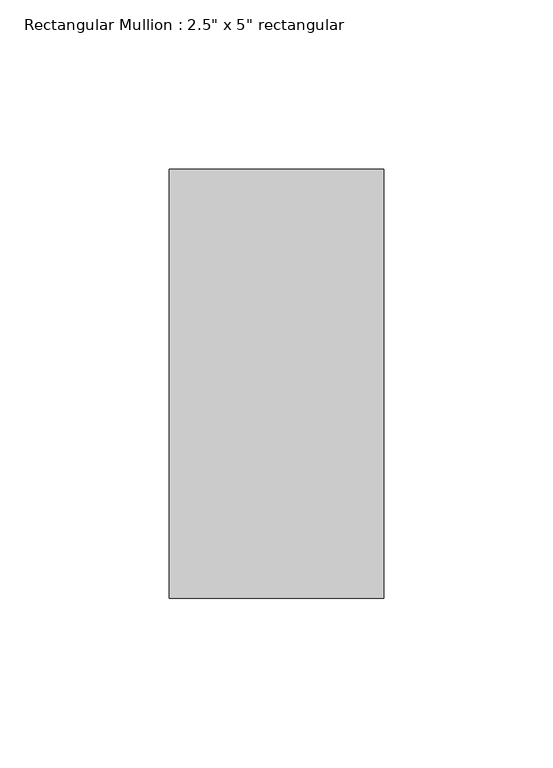
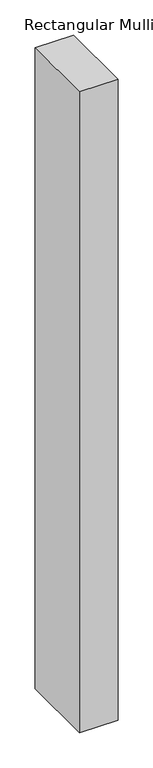
"""IFC4 building model written with IfcOpenShell, lengths in millimetres: member geometry."""

from ifc_helpers import new_model, si_unit, frame, origin, place, context, project, spatial, polyline, outline, extrude, source, transform, mapped, element, save


def member_1c5922cf(model_context):
    return source(origin(), model_context, "Body", "SweptSolid", [
        extrude(outline(polyline([(0.0, 63.5), (0.0, -63.5), (-63.5, -63.5), (-63.5, 63.5), (0.0, 63.5)])), frame((0.0, 0.0, -1116.8367632), z_axis=(0.0, 0.0, 1.0), x_axis=(1.0, 0.0, 0.0)), (0.0, 0.0, 1.0), 1116.8367632),
    ])


if __name__ == "__main__":
    model = new_model("IFC4")
    model_context = context("Model", 3, world=origin())
    ifc_project = project(units=[si_unit("LENGTHUNIT", "METRE", prefix="MILLI")], contexts=[model_context])
    site = spatial("IfcSite", under=ifc_project)
    building = spatial("IfcBuilding", under=site)
    placement = place(None, origin())
    member_shape = member_1c5922cf(model_context)
    element("IfcMember", 1, ObjectType="Rectangular Mullion : 2.5\" x 5\" rectangular", at=placement, inside=building, context=model_context, shape_type="MappedRepresentation", body=[
        mapped(member_shape, transform((0.0, 0.0, 0.0), x_axis=(1.0, 0.0, 0.0), y_axis=(0.0, 1.0, 0.0), z_axis=(0.0, 0.0, 1.0))),
    ])
    save(model, "model.ifc")

# Revit data of these elements
# Type "Rectangular Mullion : 2.5\" x 5\" rectangular"
#   built-in parameter 1007304 = 0.416667 (stored number, unit not read)
#   built-in parameter 1007301 = 0.104167 (stored number, unit not read)
#   built-in parameter 1007300 = 0.104167 (stored number, unit not read)
# Element 1 (IfcMember, "Rectangular Mullion : 2.5\" x 5\" rectangular")
#   Materials on its faces: "Aluminum"
# Materials
#   "Aluminum": class "Metal", colour RGB 247 247 247, transparency 0, Description = "Aluminum 6061", Cost = 0
